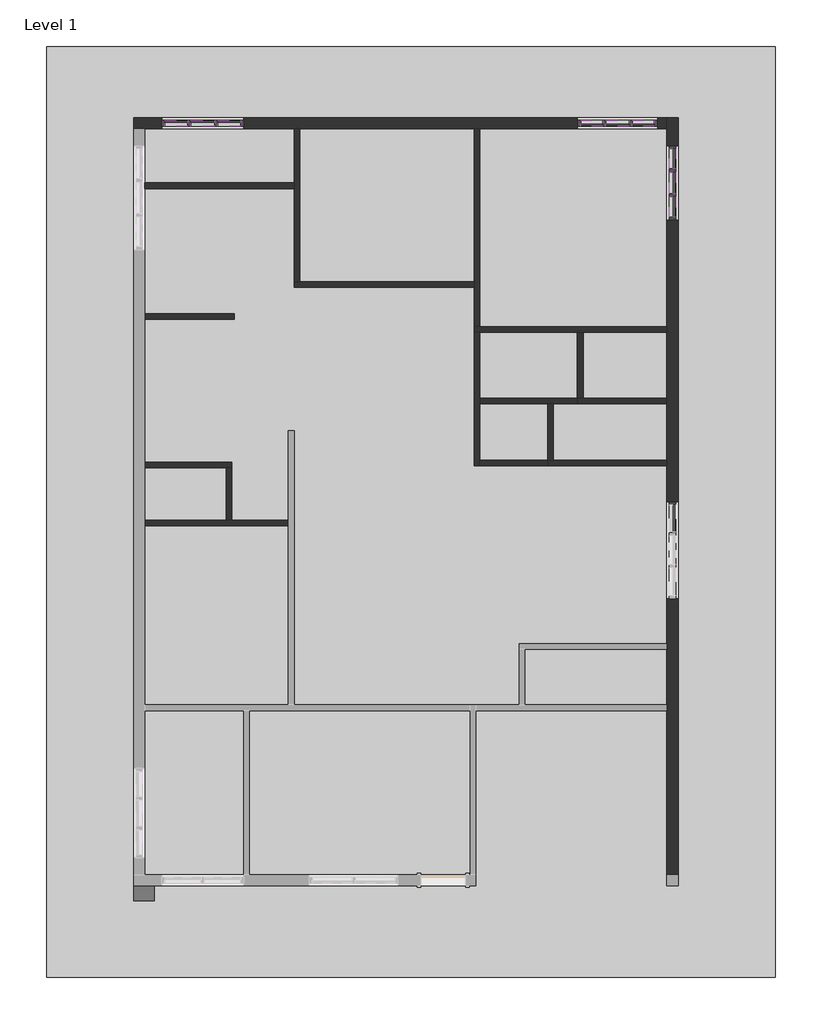
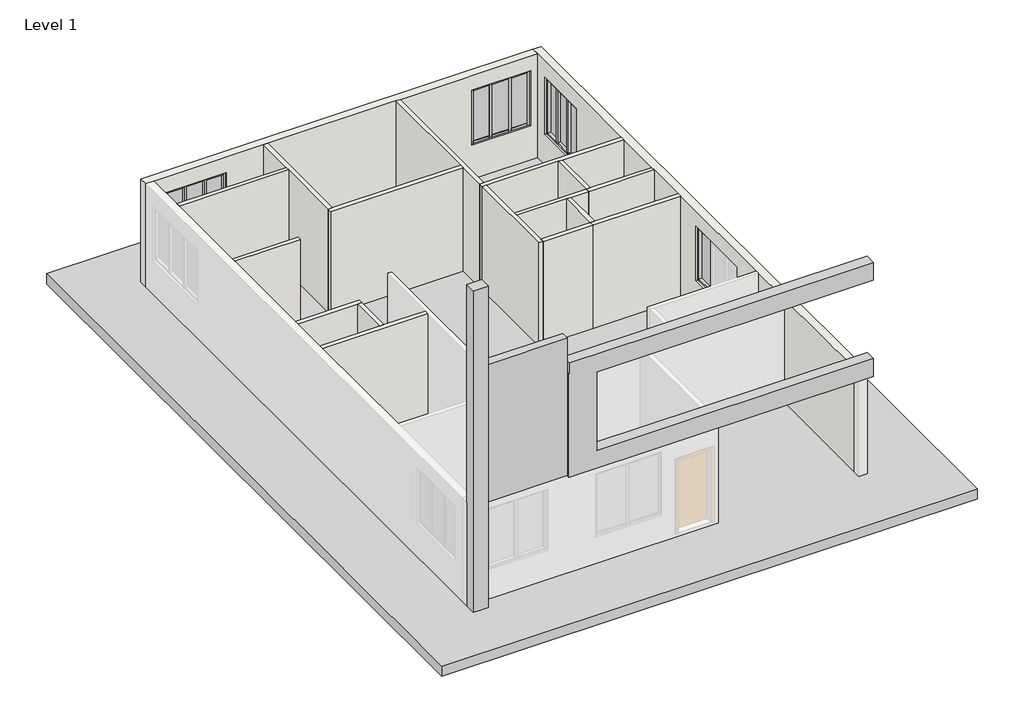
# One storey, part 2 of 2: 32 members, 18 walls, 10 plates, 2 proxies.
"""IFC4 building model written with IfcOpenShell, lengths in millimetres."""

from ifc_helpers import new_model, si_unit, origin, origin_with_axes, place, context, project, spatial, polyline, outline, extrude, faceted_brep, transform, mapped, element, save
from components import generic_models_1_generic_models_1_2a073142, generic_models_2_generic_models_2_3259aae0, member_6f432376, member_520fb4b3, member_bc7dbe04, member_dc106669, member_1f83c645, member_443975aa, member_86d06fe4, member_969ca954, member_25f01624, member_50fd6a52, member_5535eeb3, member_2ebf4a73, member_f9446df5, member_a448905b, system_panel_glazed_22e8721b, system_panel_glazed_5edd0c1a, system_panel_glazed_1157894c, system_panel_glazed_0840b29c, system_panel_glazed_6c57ad35, system_panel_glazed_545fc278, system_panel_glazed_0fd7ce52

model = new_model("IFC4")

# Units and contexts
model_context = context("Model", 3, world=origin())
ifc_project = project(units=[si_unit("LENGTHUNIT", "METRE", prefix="MILLI")], contexts=[model_context])

# Site, building, storey
site = spatial("IfcSite", under=ifc_project)
building = spatial("IfcBuilding", under=site)
storey = spatial("IfcBuildingStorey", under=building, Name="Level 1", Elevation=0.0)

# Proxies
placement = place(None, origin())
generic_models_1_generic_models_1_shape = generic_models_1_generic_models_1_2a073142(model_context)
element("IfcBuildingElementProxy", 1, Name="Generic Models 1 : Generic Models 1", ObjectType="Generic Models 1 : Generic Models 1", at=placement, inside=storey, context=model_context, shape_type="MappedRepresentation", body=[
    mapped(generic_models_1_generic_models_1_shape, transform((0.0, 0.0, 0.0), x_axis=(1.0, 0.0, 0.0), y_axis=(0.0, 1.0, 0.0), z_axis=(0.0, 0.0, 1.0))),
])
generic_models_2_generic_models_2_shape = generic_models_2_generic_models_2_3259aae0(model_context)
element("IfcBuildingElementProxy", 2, Name="Generic Models 2 : Generic Models 2", ObjectType="Generic Models 2 : Generic Models 2", at=placement, inside=storey, context=model_context, shape_type="MappedRepresentation", body=[
    mapped(generic_models_2_generic_models_2_shape, transform((0.0, 0.0, 0.0), x_axis=(1.0, 0.0, 0.0), y_axis=(0.0, 1.0, 0.0), z_axis=(0.0, 0.0, 1.0))),
])

# Members
member_shape = member_6f432376(model_context)
element("IfcMember", 3, ObjectType="Rectangular Mullion : 2.5\" x 5\" rectangular", at=placement, inside=storey, context=model_context, shape_type="MappedRepresentation", body=[
    mapped(member_shape, transform((-5990.2767684, -7548.6742702, 1004.9988244), x_axis=(0.0, 0.0, -1.0), y_axis=(-1.0, 0.0, 0.0), z_axis=(0.0, 1.0, 0.0))),
])
member_2_shape = member_520fb4b3(model_context)
element("IfcMember", 4, ObjectType="Rectangular Mullion : 2.5\" x 5\" rectangular", at=placement, inside=storey, context=model_context, shape_type="MappedRepresentation", body=[
    mapped(member_2_shape, transform((-5990.2767684, -7485.1742702, 2606.4568752), x_axis=(0.0, 1.0, 0.0), y_axis=(-1.0, 0.0, 0.0), z_axis=(0.0, 0.0, 1.0))),
])
member_3_shape = member_bc7dbe04(model_context)
element("IfcMember", 5, ObjectType="Rectangular Mullion : 2.5\" x 5\" rectangular", at=placement, inside=storey, context=model_context, shape_type="MappedRepresentation", body=[
    mapped(member_3_shape, transform((-5990.2767684, -747.8242702, 890.4108082), x_axis=(0.0, 0.0, -1.0), y_axis=(-1.0, 0.0, 0.0), z_axis=(0.0, 1.0, 0.0))),
])
member_4_shape = member_dc106669(model_context)
element("IfcMember", 6, ObjectType="Rectangular Mullion : 2.5\" x 5\" rectangular", at=placement, inside=storey, context=model_context, shape_type="MappedRepresentation", body=[
    mapped(member_4_shape, transform((-5990.2767684, -1255.8242702, 890.4108082), x_axis=(0.0, 0.0, -1.0), y_axis=(-1.0, 0.0, 0.0), z_axis=(0.0, 1.0, 0.0))),
])
element("IfcMember", 7, ObjectType="Rectangular Mullion : 2.5\" x 5\" rectangular", at=placement, inside=storey, context=model_context, shape_type="MappedRepresentation", body=[
    mapped(member_4_shape, transform((-5990.2767684, -271.5742702, 890.4108082), x_axis=(0.0, 0.0, -1.0), y_axis=(-1.0, 0.0, 0.0), z_axis=(0.0, 1.0, 0.0))),
])
member_5_shape = member_1f83c645(model_context)
element("IfcMember", 8, ObjectType="Rectangular Mullion : 2.5\" x 5\" rectangular", at=placement, inside=storey, context=model_context, shape_type="MappedRepresentation", body=[
    mapped(member_5_shape, transform((-5990.2767684, -1224.0742702, 890.4108082), x_axis=(0.0, -1.0, 0.0), y_axis=(-1.0, 0.0, 0.0), z_axis=(0.0, 0.0, -1.0))),
])
element("IfcMember", 9, ObjectType="Rectangular Mullion : 2.5\" x 5\" rectangular", at=placement, inside=storey, context=model_context, shape_type="MappedRepresentation", body=[
    mapped(member_5_shape, transform((-5990.2767684, -716.0742702, 890.4108082), x_axis=(0.0, -1.0, 0.0), y_axis=(-1.0, 0.0, 0.0), z_axis=(0.0, 0.0, -1.0))),
])
element("IfcMember", 10, ObjectType="Rectangular Mullion : 2.5\" x 5\" rectangular", at=placement, inside=storey, context=model_context, shape_type="MappedRepresentation", body=[
    mapped(member_4_shape, transform((-5990.2767684, -684.3242702, 2567.900853), x_axis=(0.0, 0.0, 1.0), y_axis=(-1.0, 0.0, 0.0), z_axis=(0.0, -1.0, 0.0))),
])
element("IfcMember", 11, ObjectType="Rectangular Mullion : 2.5\" x 5\" rectangular", at=placement, inside=storey, context=model_context, shape_type="MappedRepresentation", body=[
    mapped(member_4_shape, transform((-5990.2767684, -1668.5742702, 2567.900853), x_axis=(0.0, 0.0, 1.0), y_axis=(-1.0, 0.0, 0.0), z_axis=(0.0, -1.0, 0.0))),
])
element("IfcMember", 12, ObjectType="Rectangular Mullion : 2.5\" x 5\" rectangular", at=placement, inside=storey, context=model_context, shape_type="MappedRepresentation", body=[
    mapped(member_3_shape, transform((-5990.2767684, -1192.3242702, 2567.900853), x_axis=(0.0, 0.0, 1.0), y_axis=(-1.0, 0.0, 0.0), z_axis=(0.0, -1.0, 0.0))),
])
member_6_shape = member_443975aa(model_context)
element("IfcMember", 13, ObjectType="Rectangular Mullion : 2.5\" x 5\" rectangular", at=placement, inside=storey, context=model_context, shape_type="MappedRepresentation", body=[
    mapped(member_6_shape, transform((-5990.2767684, -208.0742702, 2567.900853), x_axis=(0.0, 1.0, 0.0), y_axis=(-1.0, 0.0, 0.0), z_axis=(0.0, 0.0, 1.0))),
])
element("IfcMember", 14, ObjectType="Rectangular Mullion : 2.5\" x 5\" rectangular", at=placement, inside=storey, context=model_context, shape_type="MappedRepresentation", body=[
    mapped(member_6_shape, transform((-5990.2767684, -1732.0742702, 890.4108082), x_axis=(0.0, -1.0, 0.0), y_axis=(-1.0, 0.0, 0.0), z_axis=(0.0, 0.0, -1.0))),
])
member_7_shape = member_86d06fe4(model_context)
element("IfcMember", 15, ObjectType="Rectangular Mullion : 2.5\" x 5\" rectangular", at=placement, inside=storey, context=model_context, shape_type="MappedRepresentation", body=[
    mapped(member_7_shape, transform((-7355.5267684, 249.1257298, 2617.6555503), x_axis=(0.0, 0.0, 1.0), y_axis=(0.0, 1.0, 0.0), z_axis=(-1.0, 0.0, 0.0))),
])
member_8_shape = member_969ca954(model_context)
element("IfcMember", 16, ObjectType="Rectangular Mullion : 2.5\" x 5\" rectangular", at=placement, inside=storey, context=model_context, shape_type="MappedRepresentation", body=[
    mapped(member_8_shape, transform((-6809.4267684, 249.1257298, 2617.6555503), x_axis=(0.0, 0.0, 1.0), y_axis=(0.0, 1.0, 0.0), z_axis=(-1.0, 0.0, 0.0))),
])
element("IfcMember", 17, ObjectType="Rectangular Mullion : 2.5\" x 5\" rectangular", at=placement, inside=storey, context=model_context, shape_type="MappedRepresentation", body=[
    mapped(member_8_shape, transform((-7869.8767684, 249.1257298, 2617.6555503), x_axis=(0.0, 0.0, 1.0), y_axis=(0.0, 1.0, 0.0), z_axis=(-1.0, 0.0, 0.0))),
])
member_9_shape = member_25f01624(model_context)
element("IfcMember", 18, ObjectType="Rectangular Mullion : 2.5\" x 5\" rectangular", at=placement, inside=storey, context=model_context, shape_type="MappedRepresentation", body=[
    mapped(member_9_shape, transform((-6841.1767684, 249.1257298, 1001.3296149), x_axis=(-1.0, 0.0, 0.0), y_axis=(0.0, 1.0, 0.0), z_axis=(0.0, 0.0, -1.0))),
])
element("IfcMember", 19, ObjectType="Rectangular Mullion : 2.5\" x 5\" rectangular", at=placement, inside=storey, context=model_context, shape_type="MappedRepresentation", body=[
    mapped(member_9_shape, transform((-7387.2767684, 249.1257298, 1001.3296149), x_axis=(-1.0, 0.0, 0.0), y_axis=(0.0, 1.0, 0.0), z_axis=(0.0, 0.0, -1.0))),
])
element("IfcMember", 20, ObjectType="Rectangular Mullion : 2.5\" x 5\" rectangular", at=placement, inside=storey, context=model_context, shape_type="MappedRepresentation", body=[
    mapped(member_8_shape, transform((-7419.0267684, 249.1257298, 1001.3296149), x_axis=(0.0, 0.0, -1.0), y_axis=(0.0, 1.0, 0.0), z_axis=(1.0, 0.0, 0.0))),
])
element("IfcMember", 21, ObjectType="Rectangular Mullion : 2.5\" x 5\" rectangular", at=placement, inside=storey, context=model_context, shape_type="MappedRepresentation", body=[
    mapped(member_8_shape, transform((-6358.5767684, 249.1257298, 1001.3296149), x_axis=(0.0, 0.0, -1.0), y_axis=(0.0, 1.0, 0.0), z_axis=(1.0, 0.0, 0.0))),
])
element("IfcMember", 22, ObjectType="Rectangular Mullion : 2.5\" x 5\" rectangular", at=placement, inside=storey, context=model_context, shape_type="MappedRepresentation", body=[
    mapped(member_7_shape, transform((-6872.9267684, 249.1257298, 1001.3296149), x_axis=(0.0, 0.0, -1.0), y_axis=(0.0, 1.0, 0.0), z_axis=(1.0, 0.0, 0.0))),
])
member_10_shape = member_50fd6a52(model_context)
element("IfcMember", 23, ObjectType="Rectangular Mullion : 2.5\" x 5\" rectangular", at=placement, inside=storey, context=model_context, shape_type="MappedRepresentation", body=[
    mapped(member_10_shape, transform((-7933.3767684, 249.1257298, 1001.3296149), x_axis=(-1.0, 0.0, 0.0), y_axis=(0.0, 1.0, 0.0), z_axis=(0.0, 0.0, -1.0))),
])
element("IfcMember", 24, ObjectType="Rectangular Mullion : 2.5\" x 5\" rectangular", at=placement, inside=storey, context=model_context, shape_type="MappedRepresentation", body=[
    mapped(member_10_shape, transform((-6295.0767684, 249.1257298, 2617.6555503), x_axis=(1.0, 0.0, 0.0), y_axis=(0.0, 1.0, 0.0), z_axis=(0.0, 0.0, 1.0))),
])
member_11_shape = member_5535eeb3(model_context)
element("IfcMember", 25, ObjectType="Rectangular Mullion : 2.5\" x 5\" rectangular", at=placement, inside=storey, context=model_context, shape_type="MappedRepresentation", body=[
    mapped(member_11_shape, transform((-15902.6267684, 249.1257298, 2586.8020872), x_axis=(0.0, 0.0, 1.0), y_axis=(0.0, -1.0, 0.0), z_axis=(1.0, 0.0, 0.0))),
])
element("IfcMember", 26, ObjectType="Rectangular Mullion : 2.5\" x 5\" rectangular", at=placement, inside=storey, context=model_context, shape_type="MappedRepresentation", body=[
    mapped(member_11_shape, transform((-14816.7767684, 249.1257298, 2586.8020872), x_axis=(0.0, 0.0, 1.0), y_axis=(0.0, -1.0, 0.0), z_axis=(1.0, 0.0, 0.0))),
])
member_12_shape = member_2ebf4a73(model_context)
element("IfcMember", 27, ObjectType="Rectangular Mullion : 2.5\" x 5\" rectangular", at=placement, inside=storey, context=model_context, shape_type="MappedRepresentation", body=[
    mapped(member_12_shape, transform((-15343.8267684, 249.1257298, 2586.8020872), x_axis=(0.0, 0.0, 1.0), y_axis=(0.0, -1.0, 0.0), z_axis=(1.0, 0.0, 0.0))),
])
member_13_shape = member_f9446df5(model_context)
element("IfcMember", 28, ObjectType="Rectangular Mullion : 2.5\" x 5\" rectangular", at=placement, inside=storey, context=model_context, shape_type="MappedRepresentation", body=[
    mapped(member_13_shape, transform((-15870.8767684, 249.1257298, 919.3492672), x_axis=(1.0, 0.0, 0.0), y_axis=(0.0, -1.0, 0.0), z_axis=(0.0, 0.0, -1.0))),
])
element("IfcMember", 29, ObjectType="Rectangular Mullion : 2.5\" x 5\" rectangular", at=placement, inside=storey, context=model_context, shape_type="MappedRepresentation", body=[
    mapped(member_13_shape, transform((-15312.0767684, 249.1257298, 919.3492672), x_axis=(1.0, 0.0, 0.0), y_axis=(0.0, -1.0, 0.0), z_axis=(0.0, 0.0, -1.0))),
])
element("IfcMember", 30, ObjectType="Rectangular Mullion : 2.5\" x 5\" rectangular", at=placement, inside=storey, context=model_context, shape_type="MappedRepresentation", body=[
    mapped(member_12_shape, transform((-15839.1267684, 249.1257298, 919.3492672), x_axis=(0.0, 0.0, -1.0), y_axis=(0.0, -1.0, 0.0), z_axis=(-1.0, 0.0, 0.0))),
])
element("IfcMember", 31, ObjectType="Rectangular Mullion : 2.5\" x 5\" rectangular", at=placement, inside=storey, context=model_context, shape_type="MappedRepresentation", body=[
    mapped(member_11_shape, transform((-15280.3267684, 249.1257298, 919.3492672), x_axis=(0.0, 0.0, -1.0), y_axis=(0.0, -1.0, 0.0), z_axis=(-1.0, 0.0, 0.0))),
])
element("IfcMember", 32, ObjectType="Rectangular Mullion : 2.5\" x 5\" rectangular", at=placement, inside=storey, context=model_context, shape_type="MappedRepresentation", body=[
    mapped(member_11_shape, transform((-16366.1767684, 249.1257298, 919.3492672), x_axis=(0.0, 0.0, -1.0), y_axis=(0.0, -1.0, 0.0), z_axis=(-1.0, 0.0, 0.0))),
])
member_14_shape = member_a448905b(model_context)
element("IfcMember", 33, ObjectType="Rectangular Mullion : 2.5\" x 5\" rectangular", at=placement, inside=storey, context=model_context, shape_type="MappedRepresentation", body=[
    mapped(member_14_shape, transform((-16429.6767684, 249.1257298, 2586.8020872), x_axis=(-1.0, 0.0, 0.0), y_axis=(0.0, -1.0, 0.0), z_axis=(0.0, 0.0, 1.0))),
])
element("IfcMember", 34, ObjectType="Rectangular Mullion : 2.5\" x 5\" rectangular", at=placement, inside=storey, context=model_context, shape_type="MappedRepresentation", body=[
    mapped(member_14_shape, transform((-14753.2767684, 249.1257298, 919.3492672), x_axis=(1.0, 0.0, 0.0), y_axis=(0.0, -1.0, 0.0), z_axis=(0.0, 0.0, -1.0))),
])

# Plates
system_panel_glazed_shape = system_panel_glazed_22e8721b(model_context)
element("IfcPlate", 35, ObjectType="System Panel : Glazed", at=placement, inside=storey, context=model_context, shape_type="MappedRepresentation", body=[
    mapped(system_panel_glazed_shape, transform((-5990.2767684, -7831.2492702, 1068.4988244), x_axis=(0.0, -1.0, 0.0), y_axis=(1.0, 0.0, 0.0), z_axis=(0.0, 0.0, 1.0))),
])
system_panel_glazed_2_shape = system_panel_glazed_5edd0c1a(model_context)
element("IfcPlate", 36, ObjectType="System Panel : Glazed", at=placement, inside=storey, context=model_context, shape_type="MappedRepresentation", body=[
    mapped(system_panel_glazed_2_shape, transform((-5990.2767684, -477.9492702, 953.9108082), x_axis=(0.0, -1.0, 0.0), y_axis=(1.0, 0.0, 0.0), z_axis=(0.0, 0.0, 1.0))),
])
element("IfcPlate", 37, ObjectType="System Panel : Glazed", at=placement, inside=storey, context=model_context, shape_type="MappedRepresentation", body=[
    mapped(system_panel_glazed_2_shape, transform((-5990.2767684, -1462.1992702, 953.9108082), x_axis=(0.0, -1.0, 0.0), y_axis=(1.0, 0.0, 0.0), z_axis=(0.0, 0.0, 1.0))),
])
system_panel_glazed_3_shape = system_panel_glazed_1157894c(model_context)
element("IfcPlate", 38, ObjectType="System Panel : Glazed", at=placement, inside=storey, context=model_context, shape_type="MappedRepresentation", body=[
    mapped(system_panel_glazed_3_shape, transform((-5990.2767684, -970.0742702, 953.9108082), x_axis=(0.0, -1.0, 0.0), y_axis=(1.0, 0.0, 0.0), z_axis=(0.0, 0.0, 1.0))),
])
system_panel_glazed_4_shape = system_panel_glazed_0840b29c(model_context)
element("IfcPlate", 39, ObjectType="System Panel : Glazed", at=placement, inside=storey, context=model_context, shape_type="MappedRepresentation", body=[
    mapped(system_panel_glazed_4_shape, transform((-6584.0017684, 249.1257298, 1064.8296149), x_axis=(-1.0, 0.0, 0.0), y_axis=(0.0, -1.0, 0.0), z_axis=(0.0, 0.0, 1.0))),
])
element("IfcPlate", 40, ObjectType="System Panel : Glazed", at=placement, inside=storey, context=model_context, shape_type="MappedRepresentation", body=[
    mapped(system_panel_glazed_4_shape, transform((-7644.4517684, 249.1257298, 1064.8296149), x_axis=(-1.0, 0.0, 0.0), y_axis=(0.0, -1.0, 0.0), z_axis=(0.0, 0.0, 1.0))),
])
system_panel_glazed_5_shape = system_panel_glazed_6c57ad35(model_context)
element("IfcPlate", 41, ObjectType="System Panel : Glazed", at=placement, inside=storey, context=model_context, shape_type="MappedRepresentation", body=[
    mapped(system_panel_glazed_5_shape, transform((-7114.2267684, 249.1257298, 1064.8296149), x_axis=(-1.0, 0.0, 0.0), y_axis=(0.0, -1.0, 0.0), z_axis=(0.0, 0.0, 1.0))),
])
system_panel_glazed_6_shape = system_panel_glazed_545fc278(model_context)
element("IfcPlate", 42, ObjectType="System Panel : Glazed", at=placement, inside=storey, context=model_context, shape_type="MappedRepresentation", body=[
    mapped(system_panel_glazed_6_shape, transform((-16134.4017684, 249.1257298, 982.8492672), x_axis=(1.0, 0.0, 0.0), y_axis=(0.0, 1.0, 0.0), z_axis=(0.0, 0.0, 1.0))),
])
element("IfcPlate", 43, ObjectType="System Panel : Glazed", at=placement, inside=storey, context=model_context, shape_type="MappedRepresentation", body=[
    mapped(system_panel_glazed_6_shape, transform((-15048.5517684, 249.1257298, 982.8492672), x_axis=(1.0, 0.0, 0.0), y_axis=(0.0, 1.0, 0.0), z_axis=(0.0, 0.0, 1.0))),
])
system_panel_glazed_7_shape = system_panel_glazed_0fd7ce52(model_context)
element("IfcPlate", 44, ObjectType="System Panel : Glazed", at=placement, inside=storey, context=model_context, shape_type="MappedRepresentation", body=[
    mapped(system_panel_glazed_7_shape, transform((-15591.4767684, 249.1257298, 982.8492672), x_axis=(1.0, 0.0, 0.0), y_axis=(0.0, 1.0, 0.0), z_axis=(0.0, 0.0, 1.0))),
])

# Walls
element("IfcWall", 45, ObjectType="4.5\"", at=placement, inside=storey, context=model_context, shape_type="Brep", body=[
    faceted_brep([(-13838.8767684, -7866.1742702, 0.0), (-14994.5767684, -7866.1742702, 0.0), (-15108.8767684, -7866.1742702, 0.0), (-16772.5767684, -7866.1742702, 0.0), (-16772.5767684, -7866.1742702, 3048.0), (-15108.8767684, -7866.1742702, 3048.0), (-14994.5767684, -7866.1742702, 3048.0), (-13838.8767684, -7866.1742702, 3048.0), (-13838.8767684, -7980.4742702, 0.0), (-13838.8767684, -7980.4742702, 3048.0), (-16772.5767684, -7980.4742702, 3048.0), (-16772.5767684, -7980.4742702, 0.0)], [[[0, 1, 2, 3, 4, 5, 6, 7]], [[8, 9, 10, 11]], [[3, 2, 1, 0, 8, 11]], [[7, 6, 5, 4, 10, 9]], [[0, 7, 9, 8]], [[4, 3, 11, 10]]]),
])
element("IfcWall", 46, ObjectType="4.5\"", at=placement, inside=storey, context=model_context, shape_type="Brep", body=[
    faceted_brep([(-6104.5767684, -3903.7742702, 0.0), (-9927.2767684, -3903.7742702, 0.0), (-10041.5767684, -3903.7742702, 0.0), (-10041.5767684, -3903.7742702, 3048.0), (-9927.2767684, -3903.7742702, 3048.0), (-6104.5767684, -3903.7742702, 3048.0), (-6104.5767684, -4018.0742702, 0.0), (-6104.5767684, -4018.0742702, 3048.0), (-7819.0767684, -4018.0742702, 3048.0), (-7933.3767684, -4018.0742702, 3048.0), (-9927.2767684, -4018.0742702, 3048.0), (-10041.5767684, -4018.0742702, 3048.0), (-10041.5767684, -4018.0742702, 0.0), (-9927.2767684, -4018.0742702, 0.0), (-7933.3767684, -4018.0742702, 0.0), (-7819.0767684, -4018.0742702, 0.0)], [[[0, 1, 2, 3, 4, 5]], [[6, 7, 8, 9, 10, 11, 12, 13, 14, 15]], [[2, 1, 0, 6, 15, 14, 13, 12]], [[5, 4, 3, 11, 10, 9, 8, 7]], [[0, 5, 7, 6]], [[3, 2, 12, 11]]]),
])
element("IfcWall", 47, ObjectType="4.5\"", at=placement, inside=storey, context=model_context, shape_type="Brep", body=[
    faceted_brep([(-9927.2767684, -3903.7742702, 0.0), (-9927.2767684, 134.8257298, 0.0), (-9927.2767684, 134.8257298, 3048.0), (-9927.2767684, -3903.7742702, 3048.0), (-10041.5767684, -3903.7742702, 0.0), (-10041.5767684, -3903.7742702, 3048.0), (-10041.5767684, -3103.6742702, 3048.0), (-10041.5767684, -2989.3742702, 3048.0), (-10041.5767684, 134.8257298, 3048.0), (-10041.5767684, 134.8257298, 0.0), (-10041.5767684, -2989.3742702, 0.0), (-10041.5767684, -3103.6742702, 0.0)], [[[0, 1, 2, 3]], [[4, 5, 6, 7, 8, 9, 10, 11]], [[1, 0, 4, 11, 10, 9]], [[3, 2, 8, 7, 6, 5]], [[0, 3, 5, 4]], [[2, 1, 9, 8]]]),
])
element("IfcWall", 48, ObjectType="4.5\"", at=placement, inside=storey, context=model_context, shape_type="Brep", body=[
    faceted_brep([(-6104.5767684, -5370.6242702, 0.0), (-7819.0767684, -5370.6242702, 0.0), (-7933.3767684, -5370.6242702, 0.0), (-7933.3767684, -5370.6242702, 3048.0), (-7819.0767684, -5370.6242702, 3048.0), (-6104.5767684, -5370.6242702, 3048.0), (-6104.5767684, -5484.9242702, 0.0), (-6104.5767684, -5484.9242702, 3048.0), (-7933.3767684, -5484.9242702, 3048.0), (-7933.3767684, -5484.9242702, 0.0)], [[[0, 1, 2, 3, 4, 5]], [[6, 7, 8, 9]], [[2, 1, 0, 6, 9]], [[5, 4, 3, 8, 7]], [[0, 5, 7, 6]], [[3, 2, 9, 8]]]),
])
element("IfcWall", 49, ObjectType="4.5\"", at=placement, inside=storey, context=model_context, shape_type="SweptSolid", body=[
    extrude(outline(polyline([(-7819.0767684, -4018.0742702), (-7819.0767684, -5370.6242702), (-7933.3767684, -5370.6242702), (-7933.3767684, -4018.0742702), (-7819.0767684, -4018.0742702)])), origin_with_axes(), (0.0, 0.0, 1.0), 3048.0),
])
element("IfcWall", 50, ObjectType="4.5\"", at=placement, inside=storey, context=model_context, shape_type="Brep", body=[
    faceted_brep([(-10041.5767684, -4018.0742702, 0.0), (-10041.5767684, -6748.5742702, 0.0), (-10041.5767684, -6748.5742702, 3048.0), (-10041.5767684, -4018.0742702, 3048.0), (-9927.2767684, -4018.0742702, 0.0), (-9927.2767684, -4018.0742702, 3048.0), (-9927.2767684, -5370.6242702, 3048.0), (-9927.2767684, -5484.9242702, 3048.0), (-9927.2767684, -6634.2742702, 3048.0), (-9927.2767684, -6748.5742702, 3048.0), (-9927.2767684, -6748.5742702, 0.0), (-9927.2767684, -6634.2742702, 0.0), (-9927.2767684, -5484.9242702, 0.0), (-9927.2767684, -5370.6242702, 0.0)], [[[0, 1, 2, 3]], [[4, 5, 6, 7, 8, 9, 10, 11, 12, 13]], [[1, 0, 4, 13, 12, 11, 10]], [[3, 2, 9, 8, 7, 6, 5]], [[0, 3, 5, 4]], [[2, 1, 10, 9]]]),
])
element("IfcWall", 51, ObjectType="4.5\"", at=placement, inside=storey, context=model_context, shape_type="Brep", body=[
    faceted_brep([(-9927.2767684, -5484.9242702, 0.0), (-8542.9767684, -5484.9242702, 0.0), (-8428.6767684, -5484.9242702, 0.0), (-7933.3767684, -5484.9242702, 0.0), (-7933.3767684, -5484.9242702, 3048.0), (-8428.6767684, -5484.9242702, 3048.0), (-8542.9767684, -5484.9242702, 3048.0), (-9927.2767684, -5484.9242702, 3048.0), (-9927.2767684, -5370.6242702, 0.0), (-9927.2767684, -5370.6242702, 3048.0), (-7933.3767684, -5370.6242702, 3048.0), (-7933.3767684, -5370.6242702, 0.0)], [[[0, 1, 2, 3, 4, 5, 6, 7]], [[8, 9, 10, 11]], [[3, 2, 1, 0, 8, 11]], [[7, 6, 5, 4, 10, 9]], [[0, 7, 9, 8]], [[4, 3, 11, 10]]]),
])
element("IfcWall", 52, ObjectType="4.5\"", at=placement, inside=storey, context=model_context, shape_type="Brep", body=[
    faceted_brep([(-6104.5767684, -6634.2742702, 0.0), (-8428.6767684, -6634.2742702, 0.0), (-8542.9767684, -6634.2742702, 0.0), (-8542.9767684, -6634.2742702, 3048.0), (-8428.6767684, -6634.2742702, 3048.0), (-6104.5767684, -6634.2742702, 3048.0), (-6104.5767684, -6748.5742702, 0.0), (-6104.5767684, -6748.5742702, 3048.0), (-8542.9767684, -6748.5742702, 3048.0), (-8542.9767684, -6748.5742702, 0.0)], [[[0, 1, 2, 3, 4, 5]], [[6, 7, 8, 9]], [[2, 1, 0, 6, 9]], [[5, 4, 3, 8, 7]], [[0, 5, 7, 6]], [[3, 2, 9, 8]]]),
])
element("IfcWall", 53, ObjectType="4.5\"", at=placement, inside=storey, context=model_context, shape_type="SweptSolid", body=[
    extrude(outline(polyline([(-8428.6767684, -5484.9242702), (-8428.6767684, -6634.2742702), (-8542.9767684, -6634.2742702), (-8542.9767684, -5484.9242702), (-8428.6767684, -5484.9242702)])), origin_with_axes(), (0.0, 0.0, 1.0), 3048.0),
])
element("IfcWall", 54, ObjectType="4.5\"", at=placement, inside=storey, context=model_context, shape_type="SweptSolid", body=[
    extrude(outline(polyline([(-8542.9767684, -6748.5742702), (-9927.2767684, -6748.5742702), (-9927.2767684, -6634.2742702), (-8542.9767684, -6634.2742702), (-8542.9767684, -6748.5742702)])), origin_with_axes(), (0.0, 0.0, 1.0), 3048.0),
])
element("IfcWall", 55, ObjectType="4.5\"", at=placement, inside=storey, context=model_context, shape_type="Brep", body=[
    faceted_brep([(-16772.5767684, -6793.0242702, 0.0), (-15108.8767684, -6793.0242702, 0.0), (-14994.5767684, -6793.0242702, 0.0), (-14994.5767684, -6793.0242702, 3048.0), (-15108.8767684, -6793.0242702, 3048.0), (-16772.5767684, -6793.0242702, 3048.0), (-16772.5767684, -6678.7242702, 0.0), (-16772.5767684, -6678.7242702, 3048.0), (-14994.5767684, -6678.7242702, 3048.0), (-14994.5767684, -6678.7242702, 0.0)], [[[0, 1, 2, 3, 4, 5]], [[6, 7, 8, 9]], [[2, 1, 0, 6, 9]], [[5, 4, 3, 8, 7]], [[0, 5, 7, 6]], [[3, 2, 9, 8]]]),
])
element("IfcWall", 56, ObjectType="4.5\"", at=placement, inside=storey, context=model_context, shape_type="SweptSolid", body=[
    extrude(outline(polyline([(-15108.8767684, -7866.1742702), (-15108.8767684, -6793.0242702), (-14994.5767684, -6793.0242702), (-14994.5767684, -7866.1742702), (-15108.8767684, -7866.1742702)])), origin_with_axes(), (0.0, 0.0, 1.0), 3048.0),
])
element("IfcWall", 57, ObjectType="4.5\"", at=placement, inside=storey, context=model_context, shape_type="SweptSolid", body=[
    extrude(outline(polyline([(-14943.7767684, -3757.7242702), (-16772.5767684, -3757.7242702), (-16772.5767684, -3643.4242702), (-14943.7767684, -3643.4242702), (-14943.7767684, -3757.7242702)])), origin_with_axes(), (0.0, 0.0, 1.0), 3048.0),
])
element("IfcWall", 58, ObjectType="4.5\"", at=placement, inside=storey, context=model_context, shape_type="SweptSolid", body=[
    extrude(outline(polyline([(-13724.5767684, -1084.3742702), (-16772.5767684, -1084.3742702), (-16772.5767684, -970.0742702), (-13724.5767684, -970.0742702), (-13724.5767684, -1084.3742702)])), origin_with_axes(), (0.0, 0.0, 1.0), 3048.0),
])
element("IfcWall", 59, ObjectType="4.5\"", at=placement, inside=storey, context=model_context, shape_type="Brep", body=[
    faceted_brep([(-13610.2767684, -2989.3742702, 0.0), (-13610.2767684, 134.8257298, 0.0), (-13610.2767684, 134.8257298, 3048.0), (-13610.2767684, -2989.3742702, 3048.0), (-13724.5767684, -2989.3742702, 0.0), (-13724.5767684, -2989.3742702, 3048.0), (-13724.5767684, -1084.3742702, 3048.0), (-13724.5767684, -970.0742702, 3048.0), (-13724.5767684, 134.8257298, 3048.0), (-13724.5767684, 134.8257298, 0.0), (-13724.5767684, -970.0742702, 0.0), (-13724.5767684, -1084.3742702, 0.0)], [[[0, 1, 2, 3]], [[4, 5, 6, 7, 8, 9, 10, 11]], [[1, 0, 4, 11, 10, 9]], [[3, 2, 8, 7, 6, 5]], [[2, 1, 9, 8]], [[0, 3, 5, 4]]]),
])
element("IfcWall", 60, ObjectType="4.5\"", at=placement, inside=storey, context=model_context, shape_type="Brep", body=[
    faceted_brep([(-10041.5767684, -2989.3742702, 0.0), (-13610.2767684, -2989.3742702, 0.0), (-13724.5767684, -2989.3742702, 0.0), (-13724.5767684, -2989.3742702, 3048.0), (-13610.2767684, -2989.3742702, 3048.0), (-10041.5767684, -2989.3742702, 3048.0), (-10041.5767684, -3103.6742702, 0.0), (-10041.5767684, -3103.6742702, 3048.0), (-13724.5767684, -3103.6742702, 3048.0), (-13724.5767684, -3103.6742702, 0.0)], [[[0, 1, 2, 3, 4, 5]], [[6, 7, 8, 9]], [[2, 1, 0, 6, 9]], [[5, 4, 3, 8, 7]], [[0, 5, 7, 6]], [[3, 2, 9, 8]]]),
])
element("IfcWall", 61, ObjectType="9\"", at=placement, inside=storey, context=model_context, shape_type="Brep", body=[
    faceted_brep([(-5875.9767684, -15105.1742702, 0.0), (-5875.9767684, 363.4257298, 0.0), (-5875.9767684, 363.4257298, 3048.0), (-5875.9767684, -15105.1742702, 3048.0), (-5875.9767684, -7485.1742702, 2606.4568752), (-5875.9767684, -7485.1742702, 1004.9988244), (-5875.9767684, -9466.3742702, 1004.9988244), (-5875.9767684, -9466.3742702, 2606.4568752), (-5875.9767684, -208.0742702, 2567.900853), (-5875.9767684, -208.0742702, 890.4108082), (-5875.9767684, -1732.0742702, 890.4108082), (-5875.9767684, -1732.0742702, 2567.900853), (-6104.5767684, 363.4257298, 0.0), (-6104.5767684, 134.8257298, 0.0), (-6104.5767684, -3903.7742702, 0.0), (-6104.5767684, -4018.0742702, 0.0), (-6104.5767684, -5370.6242702, 0.0), (-6104.5767684, -5484.9242702, 0.0), (-6104.5767684, -6634.2742702, 0.0), (-6104.5767684, -6748.5742702, 0.0), (-6104.5767684, -10387.1242702, 0.0), (-6104.5767684, -10501.4242702, 0.0), (-6104.5767684, -11638.0742702, 0.0), (-6104.5767684, -11752.3742702, 0.0), (-6104.5767684, -15105.1742702, 0.0), (-6104.5767684, -15105.1742702, 3048.0), (-6104.5767684, -11752.3742702, 3048.0), (-6104.5767684, -11638.0742702, 3048.0), (-6104.5767684, -10501.4242702, 3048.0), (-6104.5767684, -10387.1242702, 3048.0), (-6104.5767684, -6748.5742702, 3048.0), (-6104.5767684, -6634.2742702, 3048.0), (-6104.5767684, -5484.9242702, 3048.0), (-6104.5767684, -5370.6242702, 3048.0), (-6104.5767684, -4018.0742702, 3048.0), (-6104.5767684, -3903.7742702, 3048.0), (-6104.5767684, 134.8257298, 3048.0), (-6104.5767684, 363.4257298, 3048.0), (-6104.5767684, -7485.1742702, 1004.9988244), (-6104.5767684, -7485.1742702, 2606.4568752), (-6104.5767684, -9466.3742702, 2606.4568752), (-6104.5767684, -9466.3742702, 1004.9988244), (-6104.5767684, -208.0742702, 890.4108082), (-6104.5767684, -208.0742702, 2567.900853), (-6104.5767684, -1732.0742702, 2567.900853), (-6104.5767684, -1732.0742702, 890.4108082)], [[[0, 1, 2, 3], [4, 5, 6, 7], [8, 9, 10, 11]], [[12, 13, 14, 15, 16, 17, 18, 19, 20, 21, 22, 23, 24, 25, 26, 27, 28, 29, 30, 31, 32, 33, 34, 35, 36, 37], [38, 39, 40, 41], [42, 43, 44, 45]], [[1, 0, 24, 23, 22, 21, 20, 19, 18, 17, 16, 15, 14, 13, 12]], [[3, 2, 37, 36, 35, 34, 33, 32, 31, 30, 29, 28, 27, 26, 25]], [[0, 3, 25, 24]], [[2, 1, 12, 37]], [[4, 39, 38, 5]], [[39, 4, 7, 40]], [[40, 7, 6, 41]], [[5, 38, 41, 6]], [[42, 9, 8, 43]], [[43, 8, 11, 44]], [[44, 11, 10, 45]], [[9, 42, 45, 10]]]),
])
element("IfcWall", 62, ObjectType="9\"", at=placement, inside=storey, context=model_context, shape_type="Brep", body=[
    faceted_brep([(-6104.5767684, 363.4257298, 0.0), (-17001.1767684, 363.4257298, 0.0), (-17001.1767684, 363.4257298, 3048.0), (-6104.5767684, 363.4257298, 3048.0), (-6295.0767684, 363.4257298, 1001.3296149), (-6295.0767684, 363.4257298, 2617.6555503), (-7933.3767684, 363.4257298, 2617.6555503), (-7933.3767684, 363.4257298, 1001.3296149), (-16429.6767684, 363.4257298, 2586.8020872), (-16429.6767684, 363.4257298, 919.3492672), (-14753.2767684, 363.4257298, 919.3492672), (-14753.2767684, 363.4257298, 2586.8020872), (-17001.1767684, 134.8257298, 0.0), (-16772.5767684, 134.8257298, 0.0), (-13724.5767684, 134.8257298, 0.0), (-13610.2767684, 134.8257298, 0.0), (-10041.5767684, 134.8257298, 0.0), (-9927.2767684, 134.8257298, 0.0), (-6104.5767684, 134.8257298, 0.0), (-6104.5767684, 134.8257298, 3048.0), (-9927.2767684, 134.8257298, 3048.0), (-10041.5767684, 134.8257298, 3048.0), (-13610.2767684, 134.8257298, 3048.0), (-13724.5767684, 134.8257298, 3048.0), (-16772.5767684, 134.8257298, 3048.0), (-17001.1767684, 134.8257298, 3048.0), (-6295.0767684, 134.8257298, 2617.6555503), (-6295.0767684, 134.8257298, 1001.3296149), (-7933.3767684, 134.8257298, 1001.3296149), (-7933.3767684, 134.8257298, 2617.6555503), (-16429.6767684, 134.8257298, 919.3492672), (-16429.6767684, 134.8257298, 2586.8020872), (-14753.2767684, 134.8257298, 2586.8020872), (-14753.2767684, 134.8257298, 919.3492672)], [[[0, 1, 2, 3], [4, 5, 6, 7], [8, 9, 10, 11]], [[12, 13, 14, 15, 16, 17, 18, 19, 20, 21, 22, 23, 24, 25], [26, 27, 28, 29], [30, 31, 32, 33]], [[1, 0, 18, 17, 16, 15, 14, 13, 12]], [[3, 2, 25, 24, 23, 22, 21, 20, 19]], [[0, 3, 19, 18]], [[2, 1, 12, 25]], [[26, 5, 4, 27]], [[5, 26, 29, 6]], [[6, 29, 28, 7]], [[27, 4, 7, 28]], [[30, 9, 8, 31]], [[31, 8, 11, 32]], [[32, 11, 10, 33]], [[9, 30, 33, 10]]]),
])

save(model, "model.ifc")

# Revit data of these elements
# Type "Rectangular Mullion : 2.5\" x 5\" rectangular"
#   built-in parameter 1007304 = 0.416667 (stored number, unit not read)
#   built-in parameter 1007301 = 0.104167 (stored number, unit not read)
#   built-in parameter 1007300 = 0.104167 (stored number, unit not read)
# Type "System Panel : Glazed"
#   Construction Type Id = "GSP4R"
#   Analytic Construction = "1/8 in Pilkington single glazing"
#   Visual Light Transmittance = 0.9
#   Solar Heat Gain Coefficient = 0.86
#   Heat Transfer Coefficient (U) = 1.18115 BTU/(h·ft²·°F)
#   Define Thermal Properties by = 1
# Type "4.5\""
#   Assembly Code = "B2010"
#   Layers, outside or top first: 0' - 4 1/2" no material (function 1)
# Type "9\""
#   Assembly Code = "B2010"
#   Layers, outside or top first: 0' - 9" no material (function 1)
# Element 1 (IfcBuildingElementProxy, "Generic Models 1 : Generic Models 1")
#   Phase Created = New Construction
# Element 2 (IfcBuildingElementProxy, "Generic Models 2 : Generic Models 2")
#   Phase Created = New Construction
# Elements 3, 4, 5, 6, 7, 8, 9, 10, 11, 12, 13, 14, 15, 16, 17, 18, 19, 20, 21, 22, 23, 24, 25, 26, 27, 28, 29, 30, 31, 32, 33, 34 (IfcMember, "Rectangular Mullion : 2.5\" x 5\" rectangular")
#   Phase Created = New Construction
#   Materials on its faces: "Aluminum"
# Elements 35, 36, 37, 38, 39, 40, 41, 42, 43, 44 (IfcPlate, "System Panel : Glazed")
#   Phase Created = New Construction
#   Materials on its faces: "Glass"
# Elements 45, 46, 47, 48, 49, 50, 51, 52, 53, 54, 55, 56, 57, 58, 59, 60 (IfcWall, "4.5\"")
#   Top Offset = 0' - 0"
#   Base Offset = 0' - 0"
#   Unconnected Height = 10' - 0"
#   wall height = 10' - 0"
#   Phase Created = New Construction
#   Base Constraint = Level 1
#   Materials on its faces: "Default Wall"
# Elements 61, 62 (IfcWall, "9\"")
#   Top Offset = 0' - 0"
#   Base Offset = 0' - 0"
#   Unconnected Height = 10' - 0"
#   wall height = 10' - 0"
#   Phase Created = New Construction
#   Base Constraint = Level 1
#   Materials on its faces: "Default Wall"
# Materials
#   "Aluminum": class "Metal", colour RGB 247 247 247, transparency 0, Description = "Aluminum 6061", Cost = 0
#   "Glass": class "Glass", colour RGB 0 128 192, transparency 0.75, Description = "Soda Lime Glass", Cost = 0
#   "Default Wall": colour RGB 128 128 128, transparency 0, Cost = 0
